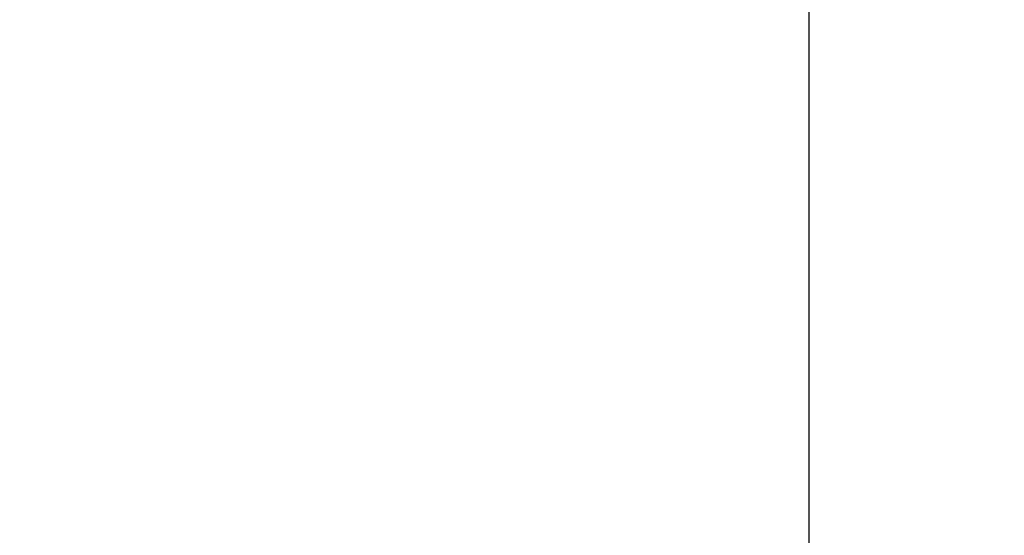
# Model space of a CAD drawing. Units: inches. Extents: x 2696 to 3240, y 1564 to 2310.
# Tile 32 of 76: x 3142.316 to 3150.171, y 1706.319 to 1710.432. Entities that reach past the tile are written whole.
import ezdxf

# ---------------------------------------------------------------- set-up
doc = ezdxf.new("R2010")
doc.units = ezdxf.units.IN
doc.layers.add('A-ANNO-DIMS', color=3, linetype='Continuous', lineweight=18)
doc.styles.add('TIMES NEW', font='times.ttf')
doc.dimstyles.new('Siddhuu', dxfattribs={"dimtxt": 6, "dimasz": 2.5, "dimexe": 1.25, "dimexo": 0.625, "dimtad": 1, "dimdec": 1, "dimlunit": 4, "dimtxsty": 'TIMES NEW', "dimcen": 2.5, "dimclrd": 256, "dimclre": 1, "dimclrt": 7, "dimadec": 0, "dimazin": 0, "dimtfac": 1, "dimtdec": 1, "dimtmove": 0, "dimatfit": 3, "dimfxl": 1, "dimtolj": 1, "dimlwd": -1, "dimarcsym": 0})

# ---------------------------------------------------------------- blocks, each defined once
blk = doc.blocks.new('*D51')
at = {"layer": 'A-ANNO-DIMS', "color": 1, "lineweight": -2, "transparency": 16777216}
for p, q in [((3016.6114, 1979.5761), (3016.6114, 1568.9511)), ((3148.6114, 1979.5761), (3148.6114, 1568.9511))]:
    blk.add_line(p, q, dxfattribs=at)
at = {"layer": 'A-ANNO-DIMS', "transparency": 16777216}
blk.add_line((3019.1114, 1570.2011), (3146.1114, 1570.2011), dxfattribs=at)
for points in [[(3019.1114, 1570.6178), (3019.1114, 1569.7844), (3016.6114, 1570.2011)], [(3146.1114, 1570.6178), (3146.1114, 1569.7844), (3148.6114, 1570.2011)]]:
    blk.add_solid(points, dxfattribs=at)
at = {"layer": 'Defpoints', "color": 0, "transparency": 16777216}
for p in [(3016.6114, 1980.2011), (3148.6114, 1980.2011), (3148.6114, 1570.2011)]:
    blk.add_point(p, dxfattribs=at)
at = {"layer": 'A-ANNO-DIMS', "color": 7, "transparency": 16777216, "insert": (3082.6114, 1573.878), "char_height": 6, "attachment_point": 5, "style": 'TIMES NEW'}
blk.add_mtext('\\A1;11\'-0"', dxfattribs=at)
blk = doc.blocks.new('*D52')
at = {"layer": 'A-ANNO-DIMS', "color": 1, "lineweight": -2, "transparency": 16777216}
for p, q in [((3148.6114, 1979.5761), (3148.6114, 1568.9511)), ((3190.6114, 1979.5761), (3190.6114, 1568.9511))]:
    blk.add_line(p, q, dxfattribs=at)
at = {"layer": 'A-ANNO-DIMS', "transparency": 16777216}
blk.add_line((3151.1114, 1570.2011), (3188.1114, 1570.2011), dxfattribs=at)
for points in [[(3151.1114, 1570.6178), (3151.1114, 1569.7844), (3148.6114, 1570.2011)], [(3188.1114, 1570.6178), (3188.1114, 1569.7844), (3190.6114, 1570.2011)]]:
    blk.add_solid(points, dxfattribs=at)
at = {"layer": 'Defpoints', "color": 0, "transparency": 16777216}
for p in [(3148.6114, 1980.2011), (3190.6114, 1980.2011), (3190.6114, 1570.2011)]:
    blk.add_point(p, dxfattribs=at)
at = {"layer": 'A-ANNO-DIMS', "color": 7, "transparency": 16777216, "insert": (3169.6114, 1573.878), "char_height": 6, "attachment_point": 5, "style": 'TIMES NEW'}
blk.add_mtext('\\A1;3\'-6"', dxfattribs=at)
blk = doc.blocks.new('*D56')
at = {"layer": 'A-ANNO-DIMS', "color": 1, "lineweight": -2, "transparency": 16777216}
for p, q in [((2966.3338, 1884.2011), (3235.8614, 1884.2011)), ((2966.3338, 1665.2011), (3235.8614, 1665.2011))]:
    blk.add_line(p, q, dxfattribs=at)
at = {"layer": 'A-ANNO-DIMS', "transparency": 16777216}
blk.add_line((3234.6114, 1667.7011), (3234.6114, 1881.7011), dxfattribs=at)
for points in [[(3234.1947, 1881.7011), (3235.0281, 1881.7011), (3234.6114, 1884.2011)], [(3234.1947, 1667.7011), (3235.0281, 1667.7011), (3234.6114, 1665.2011)]]:
    blk.add_solid(points, dxfattribs=at)
at = {"layer": 'Defpoints', "color": 0, "transparency": 16777216}
for p in [(2965.7088, 1884.2011), (3234.6114, 1884.2011), (2965.7088, 1665.2011)]:
    blk.add_point(p, dxfattribs=at)
at = {"layer": 'A-ANNO-DIMS', "color": 7, "transparency": 16777216, "insert": (3230.9345, 1774.7011), "char_height": 6, "attachment_point": 5, "rotation": 90, "style": 'TIMES NEW'}
blk.add_mtext('\\A1;18\'-3"', dxfattribs=at)

msp = doc.modelspace()

# ---------------------------------------------------------------- dimensions: what is measured, and where the dimension line sits
at = {"layer": 'A-ANNO-DIMS'}
for base, p1, p2, picture, middle in [((3148.6114, 1570.2011), (3016.6114, 1980.2011), (3148.6114, 1980.2011), '*D51', (3082.6114, 1573.878)), ((3190.6114, 1570.2011), (3148.6114, 1980.2011), (3190.6114, 1980.2011), '*D52', (3169.6114, 1573.878))]:
    dim = msp.add_linear_dim(base=base, p1=p1, p2=p2, dimstyle='Siddhuu', override={"dimdec": 1, "dimlfac": 1, "dimrnd": 0, "dimzin": 1, "dimdsep": 46, "dimlunit": 4, "dimfrac": 2}, dxfattribs=at)
    dim.commit()
    dim.dimension.update_dxf_attribs({"geometry": picture, "text_midpoint": middle})
dim = msp.add_linear_dim(base=(3234.6114, 1884.2011), p1=(2965.7088, 1665.2011), p2=(2965.7088, 1884.2011), angle=90, dimstyle='Siddhuu', override={"dimdec": 1, "dimlfac": 1, "dimrnd": 0, "dimzin": 1, "dimdsep": 46, "dimlunit": 4, "dimfrac": 2}, dxfattribs=at)
dim.commit()
dim.dimension.update_dxf_attribs({"geometry": '*D56', "text_midpoint": (3230.9345, 1774.7011)})

doc.saveas('drawing.dxf')
